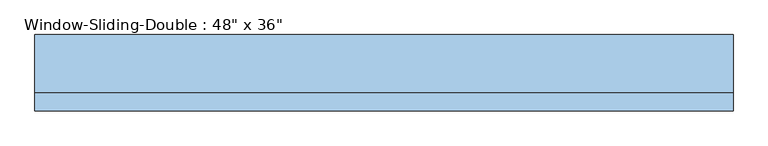
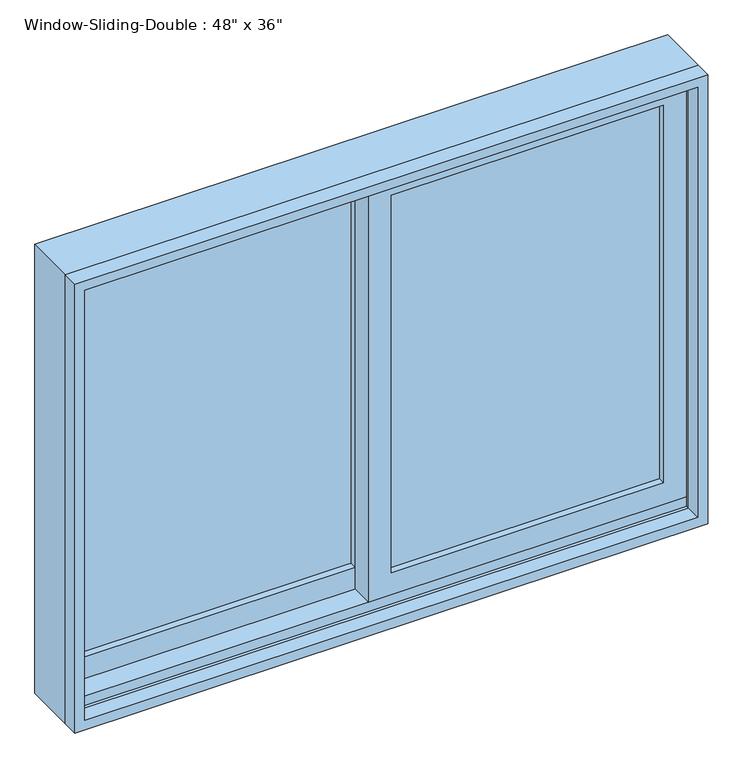
"""IFC4 building model written with IfcOpenShell, lengths in millimetres: window geometry."""

from ifc_helpers import new_model, si_unit, frame, origin, place, context, project, spatial, polyline, outline, extrude, faceted_brep, source, transform, mapped, element, save


def window_a4a981b4(model_context):
    return source(origin(), model_context, "Body", "SolidModel", [
        extrude(outline(polyline([(952.5, 590.55), (1809.75, 590.55), (1809.75, -22.225), (952.5, -22.225), (952.5, 590.55)]), holes=[polyline([(996.95, 22.225), (1765.3, 22.225), (1765.3, 546.1), (996.95, 546.1), (996.95, 22.225)])]), frame((0.0, -22.86, 0.0), z_axis=(0.0, 1.0, 0.0), x_axis=(0.0, 0.0, 1.0)), (0.0, 0.0, 1.0), 44.45),
        extrude(outline(polyline([(933.45, -590.55), (933.45, 22.225), (1809.75, 22.225), (1809.75, -590.55), (933.45, -590.55)]), holes=[polyline([(1765.3, -22.225), (996.95, -22.225), (996.95, -546.1), (1765.3, -546.1), (1765.3, -22.225)])]), frame((0.0, 21.59, 0.0), z_axis=(0.0, 1.0, 0.0), x_axis=(0.0, 0.0, 1.0)), (0.0, 0.0, 1.0), 44.45),
        extrude(outline(polyline([(-22.225, 53.34), (-22.225, 46.99), (-546.1, 46.99), (-546.1, 53.34), (-22.225, 53.34)])), frame((0.0, 0.0, 996.95), z_axis=(0.0, 0.0, 1.0), x_axis=(1.0, 0.0, 0.0)), (0.0, 0.0, 1.0), 768.35),
        extrude(outline(polyline([(-22.225, 40.64), (-22.225, 34.29), (-546.1, 34.29), (-546.1, 40.64), (-22.225, 40.64)])), frame((0.0, 0.0, 996.95), z_axis=(0.0, 0.0, 1.0), x_axis=(1.0, 0.0, 0.0)), (0.0, 0.0, 1.0), 768.35),
        extrude(outline(polyline([(546.1, 8.89), (546.1, 2.54), (22.225, 2.54), (22.225, 8.89), (546.1, 8.89)])), frame((0.0, 0.0, 996.95), z_axis=(0.0, 0.0, 1.0), x_axis=(1.0, 0.0, 0.0)), (0.0, 0.0, 1.0), 768.35),
        extrude(outline(polyline([(546.1, -3.81), (546.1, -10.16), (22.225, -10.16), (22.225, -3.81), (546.1, -3.81)])), frame((0.0, 0.0, 996.95), z_axis=(0.0, 0.0, 1.0), x_axis=(1.0, 0.0, 0.0)), (0.0, 0.0, 1.0), 768.35),
        extrude(outline(polyline([(1828.8, -609.6), (914.4, -609.6), (914.4, 609.6), (1828.8, 609.6), (1828.8, -609.6)]), holes=[polyline([(1809.75, 590.55), (933.45, 590.55), (933.45, -590.55), (1809.75, -590.55), (1809.75, 590.55)])]), frame((0.0, -60.96, 0.0), z_axis=(0.0, 1.0, 0.0), x_axis=(0.0, 0.0, 1.0)), (0.0, 0.0, 1.0), 31.75),
        faceted_brep([(-609.6, -29.21, 914.4), (-609.6, 72.39, 914.4), (609.6, 72.39, 914.4), (609.6, -29.21, 914.4), (-568.6778905, 72.39, 1787.8778905), (-568.6778905, 66.04, 1787.8778905), (-568.6778905, 66.04, 933.45), (-568.6778905, 72.39, 933.45), (568.6778905, 66.04, 1787.8778905), (568.6778905, 66.04, 933.45), (590.55, 66.04, 933.45), (590.55, 66.04, 1809.75), (-590.55, 66.04, 1809.75), (-590.55, 66.04, 933.45), (-590.55, -29.21, 1809.75), (-590.55, -29.21, 933.45), (-590.55, -22.86, 933.45), (-590.55, -22.86, 952.5), (-590.55, 21.59, 952.5), (-590.55, 21.59, 933.45), (609.6, -29.21, 1828.8), (-609.6, -29.21, 1828.8), (590.55, -29.21, 1809.75), (590.55, -29.21, 933.45), (-609.6, 72.39, 1828.8), (609.6, 72.39, 1828.8), (568.6778905, 72.39, 933.45), (568.6778905, 72.39, 1787.8778905), (590.55, 21.59, 933.45), (590.55, 21.59, 952.5), (590.55, -22.86, 952.5), (590.55, -22.86, 933.45)], [[[0, 1, 2, 3]], [[4, 5, 6, 7]], [[5, 8, 9, 10, 11, 12, 13, 6]], [[12, 14, 15, 16, 17, 18, 19, 13]], [[0, 3, 20, 21], [22, 23, 15, 14]], [[24, 1, 0, 21]], [[2, 1, 24, 25], [4, 7, 26, 27]], [[5, 4, 27, 8]], [[12, 11, 22, 14]], [[21, 20, 25, 24]], [[8, 27, 26, 9]], [[22, 11, 10, 28, 29, 30, 31, 23]], [[20, 3, 2, 25]], [[26, 7, 6, 13, 19, 28, 10, 9]], [[28, 19, 18, 29]], [[29, 18, 17, 30]], [[30, 17, 16, 31]], [[15, 23, 31, 16]]]),
    ])


if __name__ == "__main__":
    model = new_model("IFC4")
    model_context = context("Model", 3, world=origin())
    ifc_project = project(units=[si_unit("LENGTHUNIT", "METRE", prefix="MILLI")], contexts=[model_context])
    site = spatial("IfcSite", under=ifc_project)
    building = spatial("IfcBuilding", under=site)
    placement = place(None, origin())
    window_shape = window_a4a981b4(model_context)
    element("IfcWindow", 1, ObjectType="Window-Sliding-Double : 48\" x 36\"", at=placement, inside=building, context=model_context, shape_type="MappedRepresentation", body=[
        mapped(window_shape, transform((0.0, 0.0, 0.0), x_axis=(1.0, 0.0, 0.0), y_axis=(0.0, 1.0, 0.0), z_axis=(0.0, 0.0, 1.0))),
    ])
    save(model, "model.ifc")

# Revit data of these elements
# Type "Window-Sliding-Double : 48\" x 36\""
#   Type Mark = "20"
#   Fire Rating = "0.5h"
#   Assembly Code = "B2020100"
#   Analytic Construction = "Double glazing - domestic"
#   Window Inset [instance default] = 0' - 0"
#   Wall Thickness [instance default] = 0' - 6"
#   Visual Light Transmittance = 0.81
#   Thermal Resistance (R) = 1.8146 (h·ft²·°F)/BTU
#   Solar Heat Gain Coefficient = 0.76
#   Muntin Width = 1' - 8 5/8"
#   Muntin Height = 2' - 6 1/4"
#   Interior Wall Closure [instance default] = 0' - 2 3/4"
#   Heat Transfer Coefficient (U) = 0.5511 BTU/(h·ft²·°F)
#   Frame Extension [instance default] = 0' - 0 1/4"
#   Exterior Wall Closure [instance default] = 0' - 1 1/4"
#   Rough Width = 4' - 0 1/2"
#   Rough Height = 3' - 0 1/2"
#   Height = 3' - 0"
#   Extension Jamb [instance default] = 0' - 2 3/4"
#   Default Sill Height = 3' - 0"
#   Width = 4' - 0"
#   Interior Trim Visibility [instance default] = yes
#   Indicator Visibility [instance default] = yes
#   Exterior Trim Visibility [instance default] = yes
#   Muntin Visibility = yes
#   Extension Jamb Visibility [instance default] = yes
#   Muntin Pattern = Muntin Pattern_2x2 : Muntin Pattern_2x2
#   Interior Trim Material = Wood - Stained
#   Interior Trim = Trim-Window-Interior-Flat : Picture Frame
#   Interior Frame Material = Wood - Stained
#   Glass Panel Material = Glass
#   Exterior Trim Material = Clad - White
#   Exterior Trim = Trim-Window-Exterior-Flat : with Sill
#   Exterior Frame Material = Clad - White
#   Wall Closure = (empty or 0)
# Element 1 (IfcWindow, "Window-Sliding-Double : 48\" x 36\"")
#   Wall Thickness = 0' - 4 1/2"
#   Extension Jamb = 0' - 1 1/4"
#   Materials on its faces: "Wood - Stained", "Glass", "Clad - White"
# Materials
#   "Wood - Stained": class "Wood", colour RGB 224 178 126, transparency 0, Cost = 0
#   "Glass": class "Glass", colour RGB 0 128 192, transparency 0.75, Description = "Soda Lime Glass", Cost = 0
#   "Clad - White": class "Wood", colour RGB 242 242 238, transparency 0, Cost = 0
